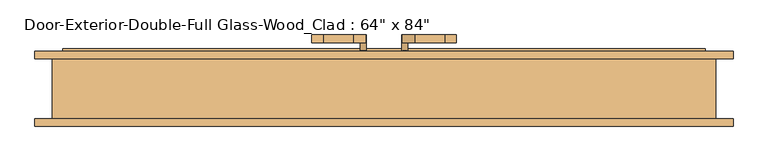
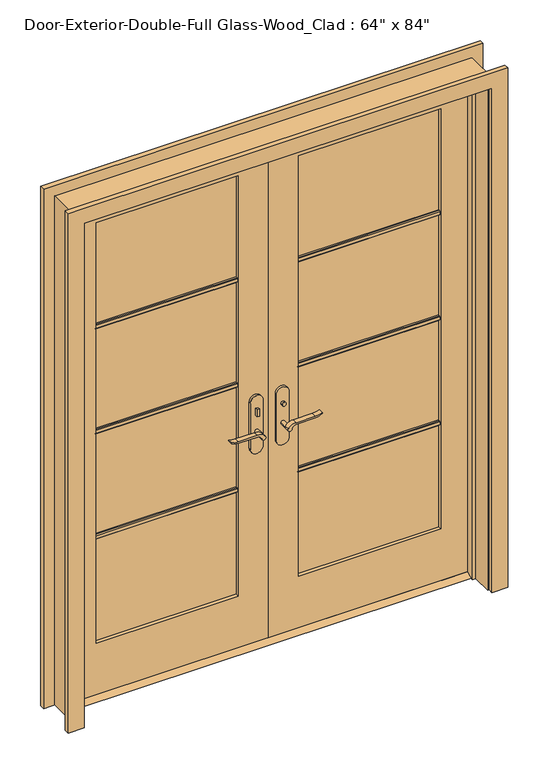
"""IFC4 building model written with IfcOpenShell, lengths in millimetres: door geometry."""

from ifc_helpers import new_model, si_unit, point, frame, frame_2d, origin, place, context, project, spatial, polyline, circle_curve, trimmed, segment, composite_curve, outline, extrude, faceted_brep, source, transform, mapped, element, save


def door_5136af5f(model_context):
    return source(origin(), model_context, "Body", "SolidModel", [
        extrude(outline(polyline([(38.1, 12.7), (73.025, 12.7), (98.425, 0.0), (12.7, 0.0), (38.1, 12.7)])), frame((-812.8, 0.0, 0.0), z_axis=(1.0, 0.0, 0.0), x_axis=(0.0, 1.0, 0.0)), (0.0, 0.0, 1.0), 1625.6),
        extrude(outline(polyline([(-47.4019111, 18.1), (-57.4019111, 18.1), (-57.4019111, 28.1), (-47.4019111, 28.1), (-47.4019111, 18.1)])), frame((0.0, 0.0, 981.9), z_axis=(0.0, 0.0, 1.0), x_axis=(1.0, 0.0, 0.0)), (0.0, 0.0, 1.0), 30.0),
        extrude(outline(composite_curve([segment(trimmed(circle_curve(frame_2d((996.9, -52.4019111)), 8.0), [point((996.9, -60.4019111))], [point((996.9, -44.4019111))], False, "CARTESIAN"), True, "CONTINUOUS"), segment(trimmed(circle_curve(frame_2d((996.9, -52.4019111)), 8.0), [point((996.9, -44.4019111))], [point((996.9, -60.4019111))], False, "CARTESIAN"), True, "CONTINUOUS")], self_intersect=False)), frame((0.0, 83.025, 0.0), z_axis=(0.0, 1.0, 0.0), x_axis=(0.0, 0.0, 1.0)), (0.0, 0.0, 1.0), 10.0),
        extrude(outline(composite_curve([segment(trimmed(circle_curve(frame_2d((897.1555521, -76.0694241)), 37.2832219), [point((919.0523287, -45.8937749))], [point((934.4, -77.7693445))], False, "CARTESIAN"), True, "CONTINUOUS"), segment(polyline([(934.4, -77.7693445), (934.4, -154.045502)]), True, "CONTINUOUS"), segment(trimmed(circle_curve(frame_2d((1017.6850638, -153.9791202)), 83.2850902), [point((934.4, -154.045502))], [point((939.4, -182.4019111))], True, "CARTESIAN"), True, "CONTINUOUS"), segment(polyline([(939.4, -182.4019111), (936.6135558, -182.4019111)]), True, "CONTINUOUS"), segment(trimmed(circle_curve(frame_2d((986.6709207, -150.4622499)), 59.3791355), [point((936.6135558, -182.4019111))], [point((927.4, -154.045502))], False, "CARTESIAN"), True, "CONTINUOUS"), segment(polyline([(927.4, -154.045502), (927.4, -77.7881013)]), True, "CONTINUOUS"), segment(trimmed(circle_curve(frame_2d((909.2738613, -77.7881013)), 18.1261387), [point((927.4, -77.7881013))], [point((914.4, -60.4019111))], True, "CARTESIAN"), True, "CONTINUOUS"), segment(trimmed(circle_curve(frame_2d((914.4, -52.4019111)), 8.0), [point((914.4, -60.4019111))], [point((919.0523287, -45.8937749))], False, "CARTESIAN"), True, "CONTINUOUS")], self_intersect=False)), frame((0.0, -21.9, 0.0), z_axis=(0.0, 1.0, 0.0), x_axis=(0.0, 0.0, 1.0)), (0.0, 0.0, 1.0), 20.0),
        extrude(outline(composite_curve([segment(trimmed(circle_curve(frame_2d((914.4, -52.4019111)), 8.0), [point((914.3999903, -60.4019111))], [point((919.0523287, -45.8937749))], False, "CARTESIAN"), True, "CONTINUOUS"), segment(trimmed(circle_curve(frame_2d((897.1555521, -76.0694241)), 37.2832219), [point((919.0523287, -45.8937749))], [point((934.4, -77.7693445))], False, "CARTESIAN"), True, "CONTINUOUS"), segment(polyline([(934.4, -77.7693445), (934.4, -154.045502)]), True, "CONTINUOUS"), segment(trimmed(circle_curve(frame_2d((1017.6850638, -153.9791202)), 83.2850902), [point((934.4, -154.045502))], [point((939.4, -182.4019111))], True, "CARTESIAN"), True, "CONTINUOUS"), segment(polyline([(939.4, -182.4019111), (936.6135558, -182.4019111)]), True, "CONTINUOUS"), segment(trimmed(circle_curve(frame_2d((986.6709207, -150.4622499)), 59.3791355), [point((936.6135558, -182.4019111))], [point((927.4, -154.045502))], False, "CARTESIAN"), True, "CONTINUOUS"), segment(polyline([(927.4, -154.045502), (927.4, -77.788099)]), True, "CONTINUOUS"), segment(trimmed(circle_curve(frame_2d((909.2738682, -77.788099)), 18.1261318), [point((927.4, -77.788099))], [point((914.3999903, -60.4019111))], True, "CARTESIAN"), True, "CONTINUOUS")], self_intersect=False)), frame((0.0, 113.025, 0.0), z_axis=(0.0, 1.0, 0.0), x_axis=(0.0, 0.0, 1.0)), (0.0, 0.0, 1.0), 20.0),
        extrude(outline(composite_curve([segment(trimmed(circle_curve(frame_2d((914.4, -52.4019111)), 8.0), [point((914.4, -60.4019111))], [point((914.4, -44.4019111))], False, "CARTESIAN"), True, "CONTINUOUS"), segment(trimmed(circle_curve(frame_2d((914.4, -52.4019111)), 8.0), [point((914.4, -44.4019111))], [point((914.4, -60.4019111))], False, "CARTESIAN"), True, "CONTINUOUS")], self_intersect=False)), frame((0.0, -1.9, 0.0), z_axis=(0.0, 1.0, 0.0), x_axis=(0.0, 0.0, 1.0)), (0.0, 0.0, 1.0), 30.0),
        extrude(outline(composite_curve([segment(trimmed(circle_curve(frame_2d((914.4, -52.4019111)), 8.0), [point((914.4, -60.4019111))], [point((914.4, -44.4019111))], False, "CARTESIAN"), True, "CONTINUOUS"), segment(trimmed(circle_curve(frame_2d((914.4, -52.4019111)), 8.0), [point((914.4, -44.4019111))], [point((914.4, -60.4019111))], False, "CARTESIAN"), True, "CONTINUOUS")], self_intersect=False)), frame((0.0, 83.025, 0.0), z_axis=(0.0, 1.0, 0.0), x_axis=(0.0, 0.0, 1.0)), (0.0, 0.0, 1.0), 30.0),
        extrude(outline(composite_curve([segment(polyline([(844.4, -27.4019111), (1039.4, -27.4019111)]), True, "CONTINUOUS"), segment(trimmed(circle_curve(frame_2d((1039.4, -52.4019111)), 25.0), [point((1039.4, -27.4019111))], [point((1039.4, -77.4019111))], False, "CARTESIAN"), True, "CONTINUOUS"), segment(polyline([(1039.4, -77.4019111), (844.4, -77.4019111)]), True, "CONTINUOUS"), segment(trimmed(circle_curve(frame_2d((844.4, -52.4019111)), 25.0), [point((844.4, -77.4019111))], [point((844.4, -27.4019111))], False, "CARTESIAN"), True, "CONTINUOUS")], self_intersect=False)), frame((0.0, 28.1, 0.0), z_axis=(0.0, 1.0, 0.0), x_axis=(0.0, 0.0, 1.0)), (0.0, 0.0, 1.0), 10.0),
        extrude(outline(composite_curve([segment(polyline([(844.4, -27.4019111), (1039.4, -27.4019111)]), True, "CONTINUOUS"), segment(trimmed(circle_curve(frame_2d((1039.4, -52.4019111)), 25.0), [point((1039.4, -27.4019111))], [point((1039.4, -77.4019111))], False, "CARTESIAN"), True, "CONTINUOUS"), segment(polyline([(1039.4, -77.4019111), (844.4, -77.4019111)]), True, "CONTINUOUS"), segment(trimmed(circle_curve(frame_2d((844.4, -52.4019111)), 25.0), [point((844.4, -77.4019111))], [point((844.4, -27.4019111))], False, "CARTESIAN"), True, "CONTINUOUS")], self_intersect=False)), frame((0.0, 73.025, 0.0), z_axis=(0.0, 1.0, 0.0), x_axis=(0.0, 0.0, 1.0)), (0.0, 0.0, 1.0), 10.0),
        extrude(outline(polyline([(47.3875, 93.025), (57.3875, 93.025), (57.3875, 83.025), (47.3875, 83.025), (47.3875, 93.025)])), frame((0.0, 0.0, 981.9), z_axis=(0.0, 0.0, 1.0), x_axis=(1.0, 0.0, 0.0)), (0.0, 0.0, 1.0), 30.0),
        extrude(outline(composite_curve([segment(trimmed(circle_curve(frame_2d((996.9, 52.3875)), 8.0), [point((996.9, 60.3875))], [point((996.9, 44.3875))], False, "CARTESIAN"), True, "CONTINUOUS"), segment(trimmed(circle_curve(frame_2d((996.9, 52.3875)), 8.0), [point((996.9, 44.3875))], [point((996.9, 60.3875))], False, "CARTESIAN"), True, "CONTINUOUS")], self_intersect=False)), frame((0.0, 18.1, 0.0), z_axis=(0.0, 1.0, 0.0), x_axis=(0.0, 0.0, 1.0)), (0.0, 0.0, 1.0), 10.0),
        extrude(outline(composite_curve([segment(trimmed(circle_curve(frame_2d((914.4, 52.3875)), 8.0), [point((919.0523287, 45.8793637))], [point((914.4, 60.3875))], False, "CARTESIAN"), True, "CONTINUOUS"), segment(trimmed(circle_curve(frame_2d((909.2738613, 77.7736901)), 18.1261387), [point((914.4, 60.3875))], [point((927.4, 77.7736901))], True, "CARTESIAN"), True, "CONTINUOUS"), segment(polyline([(927.4, 77.7736901), (927.4, 154.0310909)]), True, "CONTINUOUS"), segment(trimmed(circle_curve(frame_2d((986.6709207, 150.4478388)), 59.3791355), [point((927.4, 154.0310909))], [point((936.6135558, 182.3875))], False, "CARTESIAN"), True, "CONTINUOUS"), segment(polyline([(936.6135558, 182.3875), (939.4, 182.3875)]), True, "CONTINUOUS"), segment(trimmed(circle_curve(frame_2d((1017.6850638, 153.9647091)), 83.2850902), [point((939.4, 182.3875))], [point((934.4, 154.0310909))], True, "CARTESIAN"), True, "CONTINUOUS"), segment(polyline([(934.4, 154.0310909), (934.4, 77.7549333)]), True, "CONTINUOUS"), segment(trimmed(circle_curve(frame_2d((897.1555521, 76.0550129)), 37.2832219), [point((934.4, 77.7549333))], [point((919.0523287, 45.8793637))], False, "CARTESIAN"), True, "CONTINUOUS")], self_intersect=False)), frame((0.0, 113.025, 0.0), z_axis=(0.0, 1.0, 0.0), x_axis=(0.0, 0.0, 1.0)), (0.0, 0.0, 1.0), 20.0),
        extrude(outline(composite_curve([segment(trimmed(circle_curve(frame_2d((909.2738682, 77.7736878)), 18.1261318), [point((914.3999903, 60.3875))], [point((927.4, 77.7736878))], True, "CARTESIAN"), True, "CONTINUOUS"), segment(polyline([(927.4, 77.7736878), (927.4, 154.0310909)]), True, "CONTINUOUS"), segment(trimmed(circle_curve(frame_2d((986.6709207, 150.4478388)), 59.3791355), [point((927.4, 154.0310909))], [point((936.6135558, 182.3875))], False, "CARTESIAN"), True, "CONTINUOUS"), segment(polyline([(936.6135558, 182.3875), (939.4, 182.3875)]), True, "CONTINUOUS"), segment(trimmed(circle_curve(frame_2d((1017.6850638, 153.9647091)), 83.2850902), [point((939.4, 182.3875))], [point((934.4, 154.0310909))], True, "CARTESIAN"), True, "CONTINUOUS"), segment(polyline([(934.4, 154.0310909), (934.4, 77.7549333)]), True, "CONTINUOUS"), segment(trimmed(circle_curve(frame_2d((897.1555521, 76.0550129)), 37.2832219), [point((934.4, 77.7549333))], [point((919.0523287, 45.8793637))], False, "CARTESIAN"), True, "CONTINUOUS"), segment(trimmed(circle_curve(frame_2d((914.4, 52.3875)), 8.0), [point((919.0523287, 45.8793637))], [point((914.3999903, 60.3875))], False, "CARTESIAN"), True, "CONTINUOUS")], self_intersect=False)), frame((0.0, -21.9, 0.0), z_axis=(0.0, 1.0, 0.0), x_axis=(0.0, 0.0, 1.0)), (0.0, 0.0, 1.0), 20.0),
        extrude(outline(composite_curve([segment(trimmed(circle_curve(frame_2d((914.4, 52.3875)), 8.0), [point((914.4, 60.3875))], [point((914.4, 44.3875))], False, "CARTESIAN"), True, "CONTINUOUS"), segment(trimmed(circle_curve(frame_2d((914.4, 52.3875)), 8.0), [point((914.4, 44.3875))], [point((914.4, 60.3875))], False, "CARTESIAN"), True, "CONTINUOUS")], self_intersect=False)), frame((0.0, 83.025, 0.0), z_axis=(0.0, 1.0, 0.0), x_axis=(0.0, 0.0, 1.0)), (0.0, 0.0, 1.0), 30.0),
        extrude(outline(composite_curve([segment(trimmed(circle_curve(frame_2d((914.4, 52.3875)), 8.0), [point((914.4, 60.3875))], [point((914.4, 44.3875))], False, "CARTESIAN"), True, "CONTINUOUS"), segment(trimmed(circle_curve(frame_2d((914.4, 52.3875)), 8.0), [point((914.4, 44.3875))], [point((914.4, 60.3875))], False, "CARTESIAN"), True, "CONTINUOUS")], self_intersect=False)), frame((0.0, -1.9, 0.0), z_axis=(0.0, 1.0, 0.0), x_axis=(0.0, 0.0, 1.0)), (0.0, 0.0, 1.0), 30.0),
        extrude(outline(composite_curve([segment(trimmed(circle_curve(frame_2d((844.4, 52.3875)), 25.0), [point((844.4, 27.3875))], [point((844.4, 77.3875))], False, "CARTESIAN"), True, "CONTINUOUS"), segment(polyline([(844.4, 77.3875), (1039.4, 77.3875)]), True, "CONTINUOUS"), segment(trimmed(circle_curve(frame_2d((1039.4, 52.3875)), 25.0), [point((1039.4, 77.3875))], [point((1039.4, 27.3875))], False, "CARTESIAN"), True, "CONTINUOUS"), segment(polyline([(1039.4, 27.3875), (844.4, 27.3875)]), True, "CONTINUOUS")], self_intersect=False)), frame((0.0, 73.025, 0.0), z_axis=(0.0, 1.0, 0.0), x_axis=(0.0, 0.0, 1.0)), (0.0, 0.0, 1.0), 10.0),
        extrude(outline(composite_curve([segment(trimmed(circle_curve(frame_2d((844.4, 52.3875)), 25.0), [point((844.4, 27.3875))], [point((844.4, 77.3875))], False, "CARTESIAN"), True, "CONTINUOUS"), segment(polyline([(844.4, 77.3875), (1039.4, 77.3875)]), True, "CONTINUOUS"), segment(trimmed(circle_curve(frame_2d((1039.4, 52.3875)), 25.0), [point((1039.4, 77.3875))], [point((1039.4, 27.3875))], False, "CARTESIAN"), True, "CONTINUOUS"), segment(polyline([(1039.4, 27.3875), (844.4, 27.3875)]), True, "CONTINUOUS")], self_intersect=False)), frame((0.0, 28.1, 0.0), z_axis=(0.0, 1.0, 0.0), x_axis=(0.0, 0.0, 1.0)), (0.0, 0.0, 1.0), 10.0),
        extrude(outline(polyline([(52.07, 1578.371875), (52.07, 1559.321875), (45.72, 1559.321875), (42.545, 1562.496875), (42.545, 1575.196875), (45.72, 1578.371875), (52.07, 1578.371875)])), frame((120.65, 0.0, 0.0), z_axis=(1.0, 0.0, 0.0), x_axis=(0.0, 1.0, 0.0)), (0.0, 0.0, 1.0), 571.5),
        extrude(outline(polyline([(52.07, 1132.68125), (52.07, 1113.63125), (45.72, 1113.63125), (42.545, 1116.80625), (42.545, 1129.50625), (45.72, 1132.68125), (52.07, 1132.68125)])), frame((120.65, 0.0, 0.0), z_axis=(1.0, 0.0, 0.0), x_axis=(0.0, 1.0, 0.0)), (0.0, 0.0, 1.0), 571.5),
        extrude(outline(polyline([(52.07, 686.990625), (52.07, 667.940625), (45.72, 667.940625), (42.545, 671.115625), (42.545, 683.815625), (45.72, 686.990625), (52.07, 686.990625)])), frame((120.65, 0.0, 0.0), z_axis=(1.0, 0.0, 0.0), x_axis=(0.0, 1.0, 0.0)), (0.0, 0.0, 1.0), 571.5),
        extrude(outline(polyline([(59.055, 1578.371875), (65.405, 1578.371875), (68.58, 1575.196875), (68.58, 1562.496875), (65.405, 1559.321875), (59.055, 1559.321875), (59.055, 1578.371875)])), frame((-692.15, 0.0, 0.0), z_axis=(1.0, 0.0, 0.0), x_axis=(0.0, 1.0, 0.0)), (0.0, 0.0, 1.0), 571.5),
        extrude(outline(polyline([(59.055, 1132.68125), (65.405, 1132.68125), (68.58, 1129.50625), (68.58, 1116.80625), (65.405, 1113.63125), (59.055, 1113.63125), (59.055, 1132.68125)])), frame((-692.15, 0.0, 0.0), z_axis=(1.0, 0.0, 0.0), x_axis=(0.0, 1.0, 0.0)), (0.0, 0.0, 1.0), 571.5),
        extrude(outline(polyline([(59.055, 686.990625), (65.405, 686.990625), (68.58, 683.815625), (68.58, 671.115625), (65.405, 667.940625), (59.055, 667.940625), (59.055, 686.990625)])), frame((-692.15, 0.0, 0.0), z_axis=(1.0, 0.0, 0.0), x_axis=(0.0, 1.0, 0.0)), (0.0, 0.0, 1.0), 571.5),
        extrude(outline(polyline([(59.055, 1578.371875), (65.405, 1578.371875), (68.58, 1575.196875), (68.58, 1562.496875), (65.405, 1559.321875), (59.055, 1559.321875), (59.055, 1578.371875)])), frame((120.65, 0.0, 0.0), z_axis=(1.0, 0.0, 0.0), x_axis=(0.0, 1.0, 0.0)), (0.0, 0.0, 1.0), 571.5),
        extrude(outline(polyline([(59.055, 1132.68125), (65.405, 1132.68125), (68.58, 1129.50625), (68.58, 1116.80625), (65.405, 1113.63125), (59.055, 1113.63125), (59.055, 1132.68125)])), frame((120.65, 0.0, 0.0), z_axis=(1.0, 0.0, 0.0), x_axis=(0.0, 1.0, 0.0)), (0.0, 0.0, 1.0), 571.5),
        extrude(outline(polyline([(59.055, 686.990625), (65.405, 686.990625), (68.58, 683.815625), (68.58, 671.115625), (65.405, 667.940625), (59.055, 667.940625), (59.055, 686.990625)])), frame((120.65, 0.0, 0.0), z_axis=(1.0, 0.0, 0.0), x_axis=(0.0, 1.0, 0.0)), (0.0, 0.0, 1.0), 571.5),
        extrude(outline(polyline([(52.07, 1578.371875), (52.07, 1559.321875), (45.72, 1559.321875), (42.545, 1562.496875), (42.545, 1575.196875), (45.72, 1578.371875), (52.07, 1578.371875)])), frame((-692.15, 0.0, 0.0), z_axis=(1.0, 0.0, 0.0), x_axis=(0.0, 1.0, 0.0)), (0.0, 0.0, 1.0), 571.5),
        extrude(outline(polyline([(52.07, 1132.68125), (52.07, 1113.63125), (45.72, 1113.63125), (42.545, 1116.80625), (42.545, 1129.50625), (45.72, 1132.68125), (52.07, 1132.68125)])), frame((-692.15, 0.0, 0.0), z_axis=(1.0, 0.0, 0.0), x_axis=(0.0, 1.0, 0.0)), (0.0, 0.0, 1.0), 571.5),
        extrude(outline(polyline([(52.07, 686.990625), (52.07, 667.940625), (45.72, 667.940625), (42.545, 671.115625), (42.545, 683.815625), (45.72, 686.990625), (52.07, 686.990625)])), frame((-692.15, 0.0, 0.0), z_axis=(1.0, 0.0, 0.0), x_axis=(0.0, 1.0, 0.0)), (0.0, 0.0, 1.0), 571.5),
        extrude(outline(polyline([(0.0, 819.15), (0.0, 882.65), (2203.45, 882.65), (2203.45, -882.65), (0.0, -882.65), (0.0, -819.15), (2139.95, -819.15), (2139.95, 819.15), (0.0, 819.15)])), frame((0.0, 73.025, 0.0), z_axis=(0.0, 1.0, 0.0), x_axis=(0.0, 0.0, 1.0)), (0.0, 0.0, 1.0), 19.05),
        extrude(outline(polyline([(0.0, 819.15), (0.0, 882.65), (2203.45, 882.65), (2203.45, -882.65), (0.0, -882.65), (0.0, -819.15), (2139.95, -819.15), (2139.95, 819.15), (0.0, 819.15)])), frame((0.0, -98.425, 0.0), z_axis=(0.0, 1.0, 0.0), x_axis=(0.0, 0.0, 1.0)), (0.0, 0.0, 1.0), 19.05),
        extrude(outline(polyline([(12.7, 812.8), (2133.6, 812.8), (2133.6, 1.5875), (12.7, 1.5875), (12.7, 812.8)]), holes=[polyline([(2014.5375, 120.65), (2014.5375, 692.15), (231.775, 692.15), (231.775, 120.65), (2014.5375, 120.65)])]), frame((0.0, 38.1, 0.0), z_axis=(0.0, 1.0, 0.0), x_axis=(0.0, 0.0, 1.0)), (0.0, 0.0, 1.0), 34.925),
        extrude(outline(polyline([(2133.6, -812.8), (12.7, -812.8), (12.7, -1.6019111), (2133.6, -1.6019111), (2133.6, -812.8)]), holes=[polyline([(231.775, -692.15), (2014.5375, -692.15), (2014.5375, -120.65), (231.775, -120.65), (231.775, -692.15)])]), frame((0.0, 38.1, 0.0), z_axis=(0.0, 1.0, 0.0), x_axis=(0.0, 0.0, 1.0)), (0.0, 0.0, 1.0), 34.925),
        faceted_brep([(838.2, 73.025, 0.0), (838.2, -79.375, 0.0), (812.8, -79.375, 0.0), (812.8, 3.175, 0.0), (800.1, 3.175, 0.0), (800.1, 38.1, 0.0), (812.8, 38.1, 0.0), (812.8, 73.025, 0.0), (838.2, 73.025, 2159.0), (838.2, -79.375, 2159.0), (-838.2, -79.375, 2159.0), (-838.2, -79.375, 0.0), (-812.8, -79.375, 0.0), (-812.8, -79.375, 2133.6), (812.8, -79.375, 2133.6), (812.8, 3.175, 2133.6), (-812.8, 3.175, 2133.6), (-812.8, 3.175, 0.0), (-800.1, 3.175, 0.0), (-800.1, 3.175, 2120.9), (800.1, 3.175, 2120.9), (800.1, 38.1, 2120.9), (1.5875, 38.1, 2120.9), (-1.6019111, 38.1, 2120.9), (-800.1, 38.1, 2120.9), (-800.1, 38.1, 0.0), (-812.8, 38.1, 0.0), (-812.8, 38.1, 2133.6), (-1.6019111, 38.1, 2133.6), (1.5875, 38.1, 2133.6), (812.8, 38.1, 2133.6), (812.8, 73.025, 2133.6), (1.5875, 73.025, 2133.6), (-1.6019111, 73.025, 2133.6), (-812.8, 73.025, 2133.6), (-812.8, 73.025, 0.0), (-838.2, 73.025, 0.0), (-838.2, 73.025, 2159.0)], [[[0, 1, 2, 3, 4, 5, 6, 7]], [[1, 0, 8, 9]], [[2, 1, 9, 10, 11, 12, 13, 14]], [[3, 2, 14, 15]], [[4, 3, 15, 16, 17, 18, 19, 20]], [[5, 4, 20, 21]], [[6, 5, 21, 22, 23, 24, 25, 26, 27, 28, 29, 30]], [[7, 6, 30, 31]], [[0, 7, 31, 32, 33, 34, 35, 36, 37, 8]], [[9, 8, 37, 10]], [[14, 13, 16, 15]], [[20, 19, 24, 23, 22, 21]], [[31, 30, 29, 28, 27, 34, 33, 32]], [[12, 11, 36, 35, 26, 25, 18, 17]], [[11, 10, 37, 36]], [[13, 12, 17, 16]], [[19, 18, 25, 24]], [[27, 26, 35, 34]]]),
        extrude(outline(polyline([(692.15, 52.07), (120.65, 52.07), (120.65, 59.055), (692.15, 59.055), (692.15, 52.07)])), frame((0.0, 0.0, 231.775), z_axis=(0.0, 0.0, 1.0), x_axis=(1.0, 0.0, 0.0)), (0.0, 0.0, 1.0), 1782.7625),
        extrude(outline(polyline([(-120.65, 52.07), (-692.15, 52.07), (-692.15, 59.055), (-120.65, 59.055), (-120.65, 52.07)])), frame((0.0, 0.0, 231.775), z_axis=(0.0, 0.0, 1.0), x_axis=(1.0, 0.0, 0.0)), (0.0, 0.0, 1.0), 1782.7625),
    ])


if __name__ == "__main__":
    model = new_model("IFC4")
    model_context = context("Model", 3, world=origin())
    ifc_project = project(units=[si_unit("LENGTHUNIT", "METRE", prefix="MILLI")], contexts=[model_context])
    site = spatial("IfcSite", under=ifc_project)
    building = spatial("IfcBuilding", under=site)
    placement = place(None, origin())
    door_shape = door_5136af5f(model_context)
    element("IfcDoor", 1, ObjectType="Door-Exterior-Double-Full Glass-Wood_Clad : 64\" x 84\"", at=placement, inside=building, context=model_context, shape_type="MappedRepresentation", body=[
        mapped(door_shape, transform((0.0, 0.0, 0.0), x_axis=(1.0, 0.0, 0.0), y_axis=(0.0, 1.0, 0.0), z_axis=(0.0, 0.0, 1.0))),
    ])
    save(model, "model.ifc")

# Revit data of these elements
# Type "Door-Exterior-Double-Full Glass-Wood_Clad : 64\" x 84\""
#   Type Mark = "9"
#   Assembly Code = "B2030100"
#   Analytic Construction = "French door, wood frame with double glass"
#   Top Rail = 0' - 4 11/16"
#   Threshold Offset [instance default] = 0' - 0 1/2"
#   Thickness = 0' - 1 3/8"
#   Thermal Resistance (R) = 1.9158 (h·ft²·°F)/BTU
#   Swing Angle [instance default] = 90.00°
#   Stiles = 0' - 4 3/4"
#   Rough Width = 5' - 6"
#   Rough Height = 7' - 1"
#   Panel Width = 2' - 8"
#   Door Offset [instance default] = 0' - 0"
#   Height = 7' - 0"
#   Width = 5' - 4"
#   Heat Transfer Coefficient (U) = 0.5220 BTU/(h·ft²·°F)
#   Bottom Rail = 0' - 9 1/8"
#   Exterior Trim [instance default] = yes
#   Threshold [instance default] = yes
#   Show Grill [instance default] = yes
#   Function = 1
#   Trim Material = Cherry
#   Threshold Material = Cherry
#   Panel Material = Cherry
#   Glazing = Glass
#   Frame Material = Cherry
#   Door Handle Material = Aluminum
#   Visual Light Transmittance = 0
#   Solar Heat Gain Coefficient = 0
#   Wall Closure = (empty or 0)
#   Construction Type = (empty or 0)
# Element 1 (IfcDoor, "Door-Exterior-Double-Full Glass-Wood_Clad : 64\" x 84\"")
#   Materials on its faces: "Cherry", "Aluminum", "Glass"
# Materials
#   "Cherry": class "Wood", colour RGB 226 177 128, transparency 0, Description = "Prunus Serotina", Cost = 0
#   "Glass": class "Glass", colour RGB 0 128 192, transparency 0.75, Description = "Soda Lime Glass", Cost = 0
#   "Aluminum": class "Metal", colour RGB 247 247 247, transparency 0, Description = "Aluminum 6061", Cost = 0
